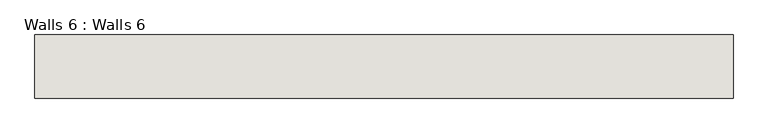
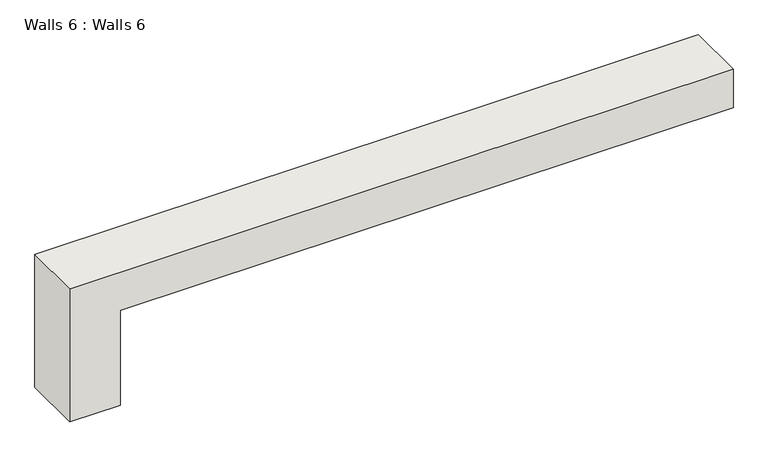
"""IFC4 building model written with IfcOpenShell, lengths in millimetres: wall geometry, Walls 6 : Walls 6."""

from ifc_helpers import new_model, si_unit, frame, origin, place, context, project, spatial, polyline, outline, extrude, source, transform, mapped, element, save


def walls_6_walls_6_9121aec3(model_context):
    return source(origin(), model_context, "Body", "SweptSolid", [
        extrude(outline(polyline([(1051.5381187, -14211.8019361), (0.0, -14211.8019361), (0.0, -13832.4019361), (746.7381187, -13832.4019361), (746.7381187, -9260.4019361), (1051.5381187, -9260.4019361), (1051.5381187, -14211.8019361)])), frame((0.0, -7417.452727, 0.0), z_axis=(0.0, 1.0, 0.0), x_axis=(0.0, 0.0, 1.0)), (0.0, 0.0, 1.0), 447.6651303),
    ])


if __name__ == "__main__":
    model = new_model("IFC4")
    model_context = context("Model", 3, world=origin())
    ifc_project = project(units=[si_unit("LENGTHUNIT", "METRE", prefix="MILLI")], contexts=[model_context])
    site = spatial("IfcSite", under=ifc_project)
    building = spatial("IfcBuilding", under=site)
    placement = place(None, origin())
    walls_6_walls_6_shape = walls_6_walls_6_9121aec3(model_context)
    element("IfcWall", 1, ObjectType="Walls 6 : Walls 6", at=placement, inside=building, context=model_context, shape_type="MappedRepresentation", body=[
        mapped(walls_6_walls_6_shape, transform((0.0, 0.0, 0.0), x_axis=(1.0, 0.0, 0.0), y_axis=(0.0, 1.0, 0.0), z_axis=(0.0, 0.0, 1.0))),
    ])
    save(model, "model.ifc")

# Revit data of these elements
# Element 1 (IfcWall, "Walls 6 : Walls 6")
#   Materials on its faces: "Default Wall"
# Materials
#   "Default Wall": colour RGB 80 80 80, transparency 0
